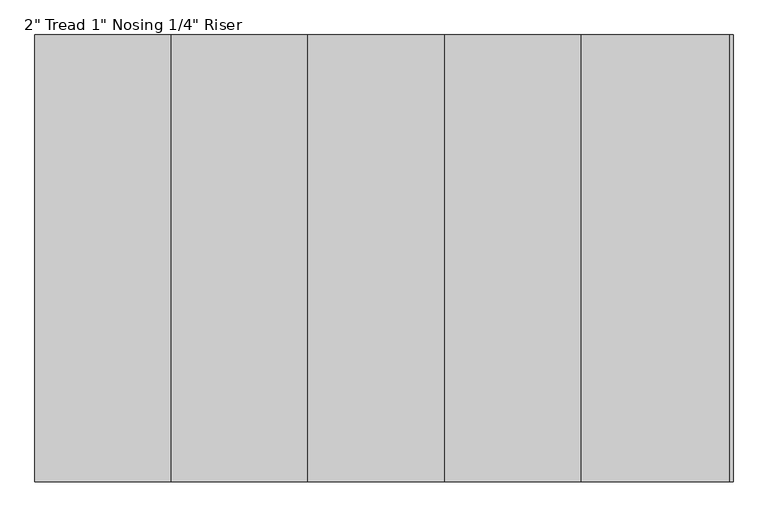
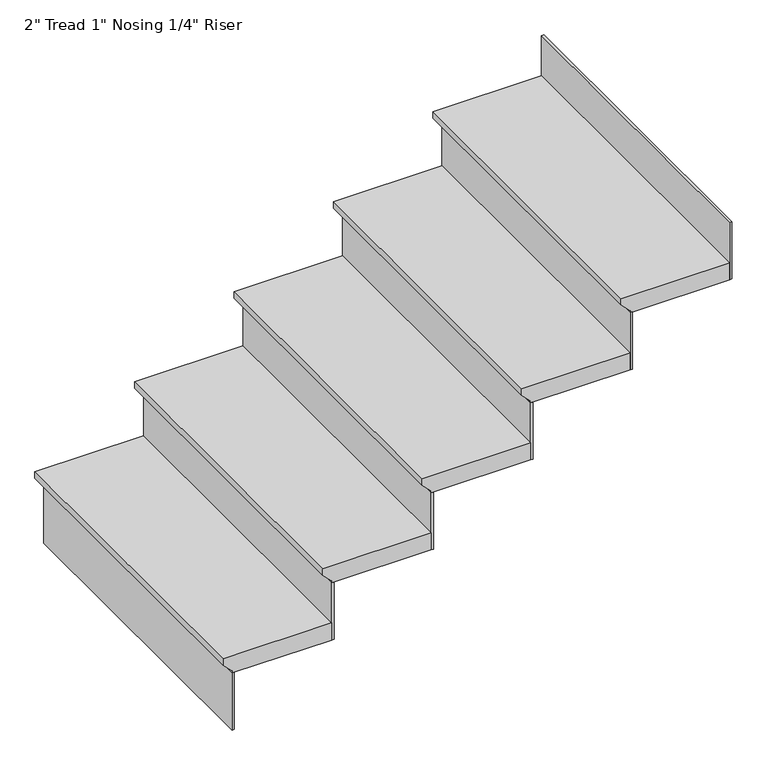
"""IFC4 building model written with IfcOpenShell, lengths in millimetres: stair flight geometry."""

from ifc_helpers import new_model, si_unit, frame, origin, place, context, project, spatial, polyline, outline, extrude, source, transform, mapped, element, save


def stair_flight_6d6c33ab(model_context):
    return source(origin(), model_context, "Body", "SweptSolid", [
        extrude(outline(polyline([(2201.3333333, -4154.1005972), (2201.3333333, -4458.9005972), (2182.2833333, -4458.9005972), (2156.8833333, -4433.5005972), (2150.5333333, -4433.5005972), (2150.5333333, -4154.1005972), (2201.3333333, -4154.1005972)])), frame((0.0, 770.2870892, 0.0), z_axis=(0.0, 1.0, 0.0), x_axis=(0.0, 0.0, 1.0)), (0.0, 0.0, 1.0), 914.4),
        extrude(outline(polyline([(-4427.1505972, 770.2870892), (-4433.5005972, 770.2870892), (-4433.5005972, 1684.6870892), (-4427.1505972, 1684.6870892), (-4427.1505972, 770.2870892)])), frame((0.0, 0.0, 1981.2), z_axis=(0.0, 0.0, 1.0), x_axis=(1.0, 0.0, 0.0)), (0.0, 0.0, 1.0), 169.3333333),
        extrude(outline(polyline([(-4147.7505972, 770.2870892), (-4154.1005972, 770.2870892), (-4154.1005972, 1684.6870892), (-4147.7505972, 1684.6870892), (-4147.7505972, 770.2870892)])), frame((0.0, 0.0, 2150.5333333), z_axis=(0.0, 0.0, 1.0), x_axis=(1.0, 0.0, 0.0)), (0.0, 0.0, 1.0), 169.3333333),
        extrude(outline(polyline([(2370.6666667, -3874.7005972), (2370.6666667, -4179.5005972), (2351.6166667, -4179.5005972), (2326.2166667, -4154.1005972), (2319.8666667, -4154.1005972), (2319.8666667, -3874.7005972), (2370.6666667, -3874.7005972)])), frame((0.0, 770.2870892, 0.0), z_axis=(0.0, 1.0, 0.0), x_axis=(0.0, 0.0, 1.0)), (0.0, 0.0, 1.0), 914.4),
        extrude(outline(polyline([(-3868.3505972, 770.2870892), (-3874.7005972, 770.2870892), (-3874.7005972, 1684.6870892), (-3868.3505972, 1684.6870892), (-3868.3505972, 770.2870892)])), frame((0.0, 0.0, 2319.8666667), z_axis=(0.0, 0.0, 1.0), x_axis=(1.0, 0.0, 0.0)), (0.0, 0.0, 1.0), 169.3333333),
        extrude(outline(polyline([(2540.0, -3595.3005972), (2540.0, -3900.1005972), (2520.95, -3900.1005972), (2495.55, -3874.7005972), (2489.2, -3874.7005972), (2489.2, -3595.3005972), (2540.0, -3595.3005972)])), frame((0.0, 770.2870892, 0.0), z_axis=(0.0, 1.0, 0.0), x_axis=(0.0, 0.0, 1.0)), (0.0, 0.0, 1.0), 914.4),
        extrude(outline(polyline([(-3588.9505972, 770.2870892), (-3595.3005972, 770.2870892), (-3595.3005972, 1684.6870892), (-3588.9505972, 1684.6870892), (-3588.9505972, 770.2870892)])), frame((0.0, 0.0, 2489.2), z_axis=(0.0, 0.0, 1.0), x_axis=(1.0, 0.0, 0.0)), (0.0, 0.0, 1.0), 169.3333333),
        extrude(outline(polyline([(2709.3333333, -3315.9005972), (2709.3333333, -3620.7005972), (2690.2833333, -3620.7005972), (2664.8833333, -3595.3005972), (2658.5333333, -3595.3005972), (2658.5333333, -3315.9005972), (2709.3333333, -3315.9005972)])), frame((0.0, 770.2870892, 0.0), z_axis=(0.0, 1.0, 0.0), x_axis=(0.0, 0.0, 1.0)), (0.0, 0.0, 1.0), 914.4),
        extrude(outline(polyline([(-3309.5505972, 770.2870892), (-3315.9005972, 770.2870892), (-3315.9005972, 1684.6870892), (-3309.5505972, 1684.6870892), (-3309.5505972, 770.2870892)])), frame((0.0, 0.0, 2658.5333333), z_axis=(0.0, 0.0, 1.0), x_axis=(1.0, 0.0, 0.0)), (0.0, 0.0, 1.0), 169.3333333),
        extrude(outline(polyline([(-3030.1505972, 770.2870892), (-3036.5005972, 770.2870892), (-3036.5005972, 1684.6870892), (-3030.1505972, 1684.6870892), (-3030.1505972, 770.2870892)])), frame((0.0, 0.0, 2827.8666667), z_axis=(0.0, 0.0, 1.0), x_axis=(1.0, 0.0, 0.0)), (0.0, 0.0, 1.0), 169.3333333),
        extrude(outline(polyline([(2878.6666667, -3036.5005972), (2878.6666667, -3341.3005972), (2859.6166667, -3341.3005972), (2834.2166667, -3315.9005972), (2827.8666667, -3315.9005972), (2827.8666667, -3036.5005972), (2878.6666667, -3036.5005972)])), frame((0.0, 770.2870892, 0.0), z_axis=(0.0, 1.0, 0.0), x_axis=(0.0, 0.0, 1.0)), (0.0, 0.0, 1.0), 914.4),
    ])


if __name__ == "__main__":
    model = new_model("IFC4")
    model_context = context("Model", 3, world=origin())
    ifc_project = project(units=[si_unit("LENGTHUNIT", "METRE", prefix="MILLI")], contexts=[model_context])
    site = spatial("IfcSite", under=ifc_project)
    building = spatial("IfcBuilding", under=site)
    placement = place(None, origin())
    stair_flight_shape = stair_flight_6d6c33ab(model_context)
    element("IfcStairFlight", 1, ObjectType="2\" Tread 1\" Nosing 1/4\" Riser", at=placement, inside=building, context=model_context, shape_type="MappedRepresentation", body=[
        mapped(stair_flight_shape, transform((0.0, 0.0, 0.0), x_axis=(1.0, 0.0, 0.0), y_axis=(0.0, 1.0, 0.0), z_axis=(0.0, 0.0, 1.0))),
    ])
    save(model, "model.ifc")

# Revit data of these elements
# Element 1 (IfcStairFlight, "2\" Tread 1\" Nosing 1/4\" Riser")
#   Materials on its faces: "Gypsum Wall Board", "Wood - Birch"
# Materials
#   "Gypsum Wall Board": class "Generic", colour RGB 127 127 127, transparency 0, Description = "Gypsum Wall Board", Cost = 0
#   "Wood - Birch": class "Wood", colour RGB 224 178 126, transparency 0
